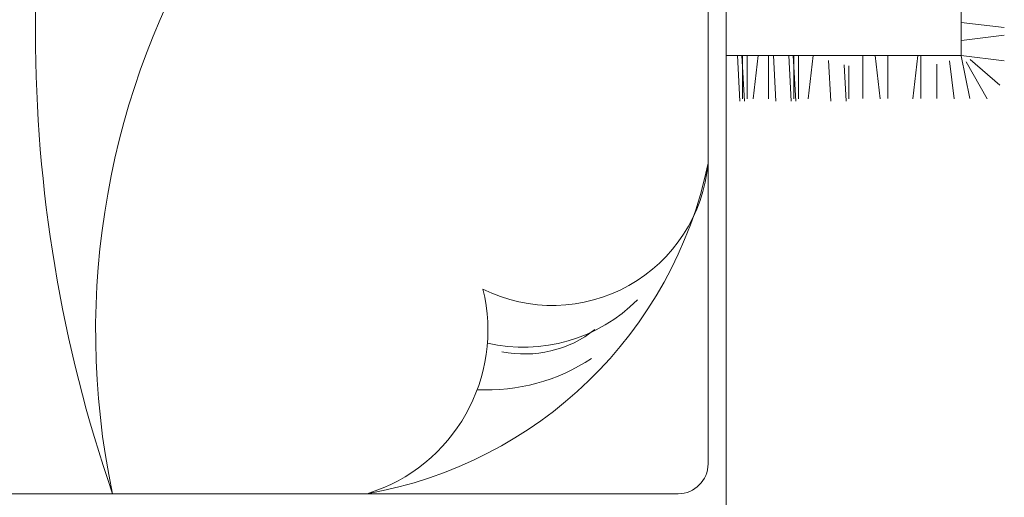
# Model space of a CAD drawing. Units: inches. Extents: x -638 to 186, y -762 to 59.
# Tile 7 of 31: x -140 to -101, y -511 to -492. Entities that reach past the tile are written whole.
import ezdxf

# ---------------------------------------------------------------- set-up
doc = ezdxf.new("R2010")
doc.units = ezdxf.units.IN
doc.layers.add('furn', color=8, linetype='Continuous', lineweight=13)

# ---------------------------------------------------------------- blocks, each defined once
blk = doc.blocks.new('BED-DOUBLE-WITH-NIGHTSTANDS')
for p, q in [((20.878, 58.468), (20.878, 13.164)), ((22.077, 11.964), (56.628, 11.964)), ((20.158, 11.244), (58.548, 11.244)), ((38.435, 1.829), (38.435, 11.244)), ((38.435, 10.789), (36.606, 10.687)), ((38.435, 10.606), (36.606, 10.504)), ((38.435, 10.585), (36.707, 10.585)), ((38.435, 10.402), (36.707, 10.402)), ((38.435, 9.957), (36.707, 10.161)), ((38.435, 9.55), (36.707, 9.55)), ((38.435, 9.347), (36.606, 9.245)), ((38.435, 8.736), (36.606, 8.634)), ((38.435, 8.553), (36.606, 8.451)), ((38.435, 8.532), (36.707, 8.532)), ((38.435, 8.349), (36.707, 8.349)), ((38.435, 7.757), (36.707, 7.961)), ((38.233, 7.135), (36.606, 7.044)), ((38.06, 6.514), (36.606, 6.433)), ((38.024, 6.332), (36.707, 6.332)), ((38.435, 5.764), (36.71, 5.764)), ((38.435, 5.274), (36.707, 5.069)), ((38.435, 4.769), (36.71, 4.769)), ((38.435, 3.565), (36.707, 3.769)), ((38.435, 3.446), (36.71, 3.446)), ((38.086, 2.81), (36.71, 2.81)), ((38.221, 2.295), (36.707, 2.115)), ((38.185, 1.631), (36.707, 0.792)), ((38.421, 1.829), (36.71, 1.486)), ((38.435, 1.829), (38.231, 0.102)), ((68.982, 1.829), (38.435, 1.829)), ((39.046, 1.815), (39.249, 0.102)), ((39.759, 1.829), (39.555, 0.102)), ((38.274, 1.47), (37.248, 0.275))]:
    blk.add_line(p, q)
for centre, radius, start, end in [((39.353, -18.016), 56.914, 71.0577, 108.9423), ((27.358, 4.824), 31.662, 15.7708, 101.8099), ((37.529, 28.521), 16.903, 189.9106, 258.3834), ((27.435, 27.646), 6.865, 197.236, 283.8635), ((32.674, 20.841), 7.64, 177.2247, 213.4103), ((34.672, 18.19), 6.25, 153.4835, 264.9765), ((33.202, 19.362), 6.454, 167.1156, 225.1048), ((30.992, 19.307), 4.516, 168.3591, 218.5338), ((22.077, 13.164), 1.2, 180, 270)]:
    blk.add_arc(centre, radius, start, end)

msp = doc.modelspace()

# ---------------------------------------------------------------- block references
at = {"layer": 'furn', "rotation": 90.00000000000017}
msp.add_blockref('BED-DOUBLE-WITH-NIGHTSTANDS', (-100.575, -532.203), dxfattribs=at)

doc.saveas('drawing.dxf')
